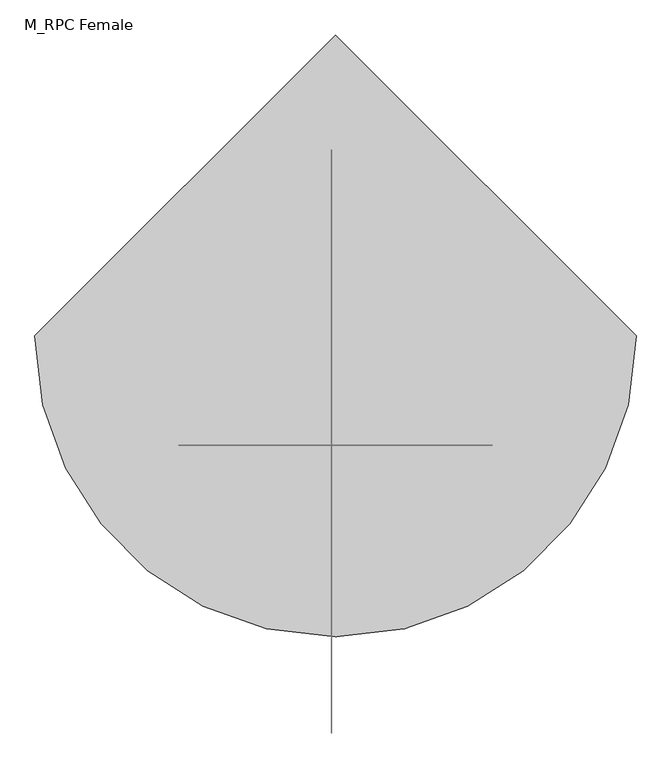
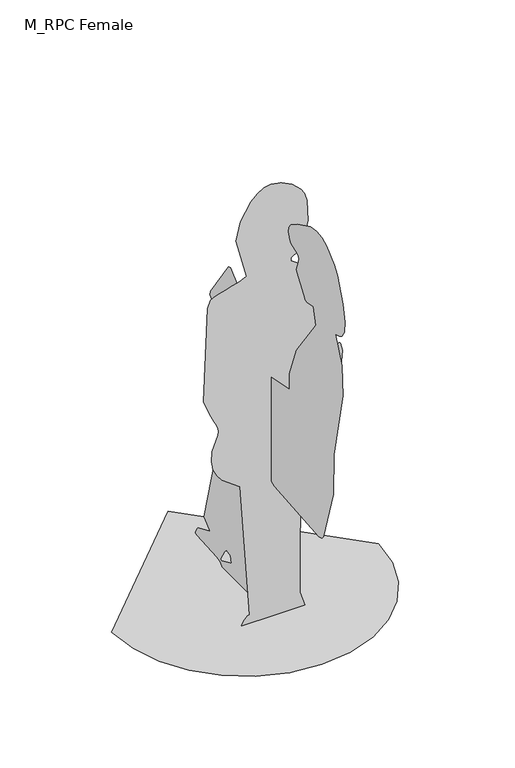
"""IFC4 building model written with IfcOpenShell, lengths in millimetres: proxy geometry, M_RPC Female."""

from ifc_helpers import new_model, si_unit, origin, place, context, project, spatial, triangles, source, transform, mapped, element, save


def m_rpc_female_e5f04239(model_context):
    return source(origin(), model_context, "Body", "Tessellation", [
        triangles([(-437.3057565, 0.0, 2.93e-05), (-425.7448342, -100.2015691, 2.93e-05), (-392.8194094, -192.2206799, 2.93e-05), (-341.1658762, -273.4208834, 2.93e-05), (-273.4209015, -341.1659489, 2.93e-05), (-192.2206254, -392.819373, 2.93e-05), (-100.2015237, -425.7447979, 2.93e-05), (1.91e-05, -437.3057565, 2.93e-05), (100.2015782, -425.7448342, 2.93e-05), (192.220698, -392.8194094, 2.93e-05), (273.4209015, -341.1658762, 2.93e-05), (341.1660215, -273.4209015, 2.93e-05), (392.819373, -192.2206072, 2.93e-05), (425.7447979, -100.2014965, 2.93e-05), (437.3057565, 3.36e-05, 2.93e-05), (-5.73e-05, 437.3057928, 2.93e-05), (-5.5814555, 72.246871, 69.496344), (-5.5814561, 67.031142, 46.0256608), (-5.5814583, 124.4039254, 19.9471336), (-5.5814583, 129.6196318, 25.1628196), (-5.5814566, 107.6002273, 62.2269385), (-5.5814561, 95.7175496, 74.7120321), (-5.5814561, -28.6037069, 4.4e-06), (-5.5814555, -39.8908654, 35.5942482), (-5.5814555, -42.4985551, 37.2668205), (-5.5814544, -45.6385706, 39.1828009), (-5.5814544, -48.9915363, 41.1595652), (-5.5814544, -52.2381223, 43.0148345), (-5.5814544, -55.0589122, 44.56573), (-5.5814544, -57.1346076, 45.6302408), (-5.5814544, -58.1458059, 46.0256654), (-5.5814555, -58.1458876, 5.3e-06), (-5.5814555, -108.9534241, 6.8e-06), (-5.5814544, -116.5758149, 29.8220214), (-5.5814504, -109.3236867, 163.616957), (-5.5814413, -45.457159, 488.7457126), (-5.5814407, -47.714434, 510.223653), (-5.5814407, -52.9301222, 512.8314517), (-5.5814407, -176.6935208, 461.1352976), (-5.5814373, -431.0100652, 441.4516517), (-5.5814373, -446.7160832, 445.0273055), (-5.5814368, -456.1585665, 455.8251566), (-5.58143, -511.6809405, 636.0529638), (-5.581426, -514.5203021, 776.2247131), (-5.5814186, -566.7671494, 1012.4528812), (-5.5814158, -561.4616592, 1112.6378271), (-5.5814129, -522.3438071, 1198.6970364), (-5.5814129, -544.7658397, 1204.5966036), (-5.5814118, -561.2097487, 1214.9815075), (-5.5814118, -573.9143148, 1236.2570984), (-5.5814101, -577.4586843, 1272.8740494), (-5.5814084, -566.4219306, 1329.2825249), (-5.5814067, -535.3830912, 1409.9332706), (-5.5814067, -516.7872059, 1433.7636475), (-5.5814055, -472.5754423, 1474.3204742), (-5.5814055, -445.9832065, 1486.7813416), (-5.5814067, -415.7490417, 1491.1880493), (-5.5814067, -381.3846422, 1485.4068615), (-5.5814084, -308.1102631, 1450.1703495), (-5.5814101, -271.6907746, 1426.3735462), (-5.5814107, -259.9822778, 1410.5514015), (-5.5814118, -256.5008769, 1391.3528641), (-5.5814118, -264.1662884, 1368.2074745), (-5.5814118, -270.5525991, 1361.5164585), (-5.5814118, -307.4893707, 1345.9730759), (-5.5814118, -313.6895373, 1341.0963387), (-5.5814118, -316.3233519, 1334.3053288), (-5.5814129, -314.5104538, 1321.5896805), (-5.5814141, -303.2841405, 1289.971843), (-5.5814141, -303.9328654, 1281.3184467), (-5.5814146, -344.8551496, 1227.4567635), (-5.5814158, -350.2254976, 1216.9519541), (-5.5814158, -354.0100413, 1213.137216), (-5.5814158, -360.9104559, 1211.8311184), (-5.5814146, -397.1668911, 1216.9519541), (-5.5814158, -412.8139375, 1162.1870556), (-5.581422, -300.7217424, 1007.464959), (-5.581426, -262.9222146, 903.7019611), (-5.5814277, -261.5584715, 849.2446747), (-5.58143, -151.2454102, 828.1022152), (-5.58143, -131.1657765, 828.3817766), (-5.5814288, -146.9133073, 873.4847649), (-5.5814288, -146.8129046, 875.3230974), (-5.5814288, -136.5283852, 880.5989382), (-5.581426, 66.2908528, 1062.7618744), (-5.581426, 72.9541861, 1068.1172161), (-5.5814266, 85.3175848, 1063.7719145), (-5.5814322, 186.9119923, 916.7356859), (-5.5814328, 189.6002729, 904.0095005), (-5.5814339, 74.8547106, 802.3032812), (-5.5814345, 53.5231683, 768.5290346), (-5.5814345, 40.9526102, 757.9697954), (-5.5814345, 7.0502408, 750.1462177), (-5.5814362, -30.7395663, 681.3427139), (-5.5814362, -32.0672787, 677.1262562), (-5.5814368, -2.7970168, 673.1418337), (-5.5814379, 74.8547106, 666.6947708), (-5.5814566, 223.5023279, 113.8298615), (-5.5814572, 192.3027606, 86.4272282), (-5.5814572, 189.6002729, 82.5355962), (-5.5814595, 257.4045281, 53.849234), (-5.5814595, 261.0572667, 50.6335418), (-5.5814595, 266.9932234, 41.9573409), (-5.58146, 270.4022813, 33.1798288), (-5.58146, 270.8965462, 29.8373185), (-5.58146, 270.443685, 27.7706614), (-5.58146, 262.21192, 24.6723971), (-5.5814583, 148.3989361, 17.7234776), (-5.5814583, 129.6196318, 12.1235594), (-5.5814583, 119.2279423, 0.0), (-103.2161017, -158.8625416, 3.138314), (-93.5649194, -158.8625416, 19.242982), (-88.6211895, -158.8625416, 24.4594286), (-82.9717796, -158.8625416, 28.4095146), (-76.7113605, -158.8625416, 30.3784918), (-108.0056168, -158.8625779, 484.1449396), (-166.5178156, -158.8625779, 527.9969504), (-183.6322324, -158.8625779, 549.73316), (-196.1559229, -158.8625779, 575.232294), (-202.0512208, -158.8625779, 604.6166196), (-199.2805142, -158.8625779, 638.0082951), (-180.7337175, -158.8625779, 688.9249546), (-179.5104455, -158.8625779, 700.1737593), (-181.025542, -158.8625779, 711.0281839), (-186.0298695, -158.8625779, 724.8027792), (-192.7431225, -158.8625779, 739.7135696), (-208.5562016, -158.8625779, 771.7149593), (-227.9668809, -158.8625779, 820.5580536), (-215.5926726, -158.8626143, 1139.7189503), (-204.4961842, -158.8626143, 1164.7947453), (-195.70417, -158.8626143, 1170.2244284), (-178.399812, -158.8626143, 1176.5899555), (-156.0960135, -158.8626143, 1183.4364126), (-132.3055416, -158.8626143, 1190.3077229), (-110.5413086, -158.8626143, 1196.7492628), (-94.3160908, -158.8626143, 1202.3054644), (-87.1427823, -158.8626143, 1206.520396), (-121.0448735, -158.8626143, 1339.5209988), (-105.9598205, -158.8626324, 1402.4766037), (-72.2006347, -158.8626324, 1459.392897), (-51.1398926, -158.8626324, 1480.6086079), (-28.7965572, -158.8626324, 1494.3413452), (-6.2993123, -158.8626324, 1498.5999516), (28.3785935, -158.8626324, 1491.3003971), (62.9443729, -158.8626324, 1473.3395748), (92.2084342, -158.8626324, 1445.5309525), (103.2305721, -158.8626324, 1428.1879704), (112.1216355, -158.8626324, 1400.9896305), (114.2135136, -158.8626143, 1329.2264236), (96.1614451, -158.8626143, 1258.9092041), (79.8725593, -158.8626143, 1233.5183121), (58.89705, -158.8626143, 1219.5597164), (58.89705, -158.8626143, 1209.128231), (105.4402574, -158.8626143, 1177.1569994), (186.6818646, -158.8626143, 1146.5396822), (190.9101676, -158.8626143, 1130.2527403), (197.4604945, -158.8625961, 874.5614433), (217.1152177, -158.8625961, 870.6124111), (219.4354431, -158.8625961, 869.5266489), (221.3548754, -158.8625961, 866.986179), (227.9668991, -158.8625779, 839.7665468), (217.9761209, -158.8625779, 726.675412), (216.778683, -158.8625779, 725.536964), (198.418848, -158.8625779, 721.3532078), (197.1132955, -158.8625779, 721.4596693), (188.2934486, -158.8625779, 736.0850121), (176.2504519, -158.8625779, 750.1460724), (172.5434834, -158.8625779, 744.3784012), (169.4576071, -158.8625779, 737.6237263), (166.7654749, -158.8625779, 730.2867468), (164.2397206, -158.8625779, 722.7717985), (161.6530689, -158.8625779, 715.4834352), (158.7781536, -158.8625779, 708.8262835), (155.3876265, -158.8625779, 703.2046789), (164.598783, -158.8625779, 582.3864721), (159.7288041, -158.8625779, 557.993666), (150.1719383, -158.8625779, 536.3020758), (143.4521541, -158.8625779, 528.6086137), (105.433708, -158.8625779, 509.5447337), (96.8765541, -158.8625779, 503.2554737), (90.1912608, -158.8625779, 494.5763523), (88.7455914, -158.8625416, 49.4103652), (105.4366057, -158.8625416, 7.4e-05), (-104.3910027, -158.8625416, 7.4e-05)], [[15, 16, 1], [14, 15, 1], [14, 1, 2], [13, 14, 2], [13, 2, 3], [13, 3, 4], [12, 13, 4], [11, 12, 4], [11, 4, 5], [11, 5, 6], [11, 6, 7], [11, 7, 8], [11, 8, 9], [11, 9, 10], [23, 17, 18], [110, 23, 18], [110, 18, 19], [109, 110, 19], [17, 23, 24], [31, 32, 33], [31, 33, 34], [109, 19, 20], [108, 109, 20], [88, 89, 90], [82, 83, 84], [85, 86, 87], [105, 106, 107], [104, 105, 107], [103, 104, 107], [102, 103, 107], [101, 102, 107], [100, 101, 107], [100, 107, 108], [100, 108, 20], [100, 20, 21], [100, 21, 22], [87, 88, 90], [85, 87, 90], [84, 85, 90], [84, 90, 91], [84, 91, 92], [84, 92, 93], [82, 84, 93], [81, 82, 93], [81, 93, 94], [80, 81, 94], [80, 94, 95], [99, 100, 22], [17, 24, 25], [17, 25, 26], [31, 34, 35], [30, 31, 35], [17, 26, 27], [17, 27, 28], [17, 28, 29], [29, 30, 35], [17, 29, 35], [22, 17, 35], [99, 22, 35], [98, 99, 35], [97, 98, 35], [97, 35, 36], [97, 36, 37], [96, 97, 37], [96, 37, 38], [95, 96, 38], [80, 95, 38], [80, 38, 39], [79, 80, 39], [79, 39, 40], [79, 40, 41], [79, 41, 42], [79, 42, 43], [79, 43, 44], [78, 79, 44], [77, 78, 44], [77, 44, 45], [77, 45, 46], [76, 77, 46], [76, 46, 47], [75, 76, 47], [72, 73, 74], [71, 72, 74], [61, 62, 63], [60, 61, 63], [60, 63, 64], [59, 60, 64], [59, 64, 65], [59, 65, 66], [58, 59, 66], [57, 58, 66], [56, 57, 66], [55, 56, 66], [54, 55, 66], [54, 66, 67], [53, 54, 67], [52, 53, 67], [52, 67, 68], [51, 52, 68], [50, 51, 68], [49, 50, 68], [48, 49, 68], [47, 48, 68], [75, 47, 68], [74, 75, 68], [71, 74, 68], [70, 71, 68], [69, 70, 68], [183, 184, 111], [183, 111, 112], [183, 112, 113], [183, 113, 114], [183, 114, 115], [182, 183, 115], [181, 182, 115], [181, 115, 116], [154, 155, 156], [164, 165, 166], [180, 181, 116], [163, 164, 166], [162, 163, 166], [162, 166, 167], [161, 162, 167], [160, 161, 167], [159, 160, 167], [158, 159, 167], [157, 158, 167], [180, 116, 117], [180, 117, 118], [180, 118, 119], [180, 119, 120], [180, 120, 121], [180, 121, 122], [179, 180, 122], [179, 122, 123], [178, 179, 123], [177, 178, 123], [176, 177, 123], [175, 176, 123], [174, 175, 123], [174, 123, 124], [174, 124, 125], [173, 174, 125], [172, 173, 125], [171, 172, 125], [170, 171, 125], [169, 170, 125], [169, 125, 126], [168, 169, 126], [168, 126, 127], [167, 168, 127], [157, 167, 127], [157, 127, 128], [156, 157, 128], [154, 156, 128], [153, 154, 128], [153, 128, 129], [153, 129, 130], [153, 130, 131], [153, 131, 132], [153, 132, 133], [153, 133, 134], [153, 134, 135], [153, 135, 136], [153, 136, 137], [152, 153, 137], [151, 152, 137], [150, 151, 137], [149, 150, 137], [149, 137, 138], [149, 138, 139], [148, 149, 139], [147, 148, 139], [146, 147, 139], [146, 139, 140], [145, 146, 140], [145, 140, 141], [144, 145, 141], [144, 141, 142], [144, 142, 143]], closed=False),
    ])


if __name__ == "__main__":
    model = new_model("IFC4")
    model_context = context("Model", 3, world=origin())
    ifc_project = project(units=[si_unit("LENGTHUNIT", "METRE", prefix="MILLI")], contexts=[model_context])
    site = spatial("IfcSite", under=ifc_project)
    building = spatial("IfcBuilding", under=site)
    placement = place(None, origin())
    m_rpc_female_shape = m_rpc_female_e5f04239(model_context)
    element("IfcBuildingElementProxy", 1, Name="M_RPC Female", ObjectType="M_RPC Female", at=placement, inside=building, context=model_context, shape_type="MappedRepresentation", body=[
        mapped(m_rpc_female_shape, transform((0.0, 0.0, 0.0), x_axis=(1.0, 0.0, 0.0), y_axis=(0.0, 1.0, 0.0), z_axis=(0.0, 0.0, 1.0))),
    ])
    save(model, "model.ifc")

# Revit data of these elements
# Type "M_RPC Female"
#   built-in parameter 1005195 = "RPC-8-FXA2-QQQ0-UGV2-6"
#   Height = 0
